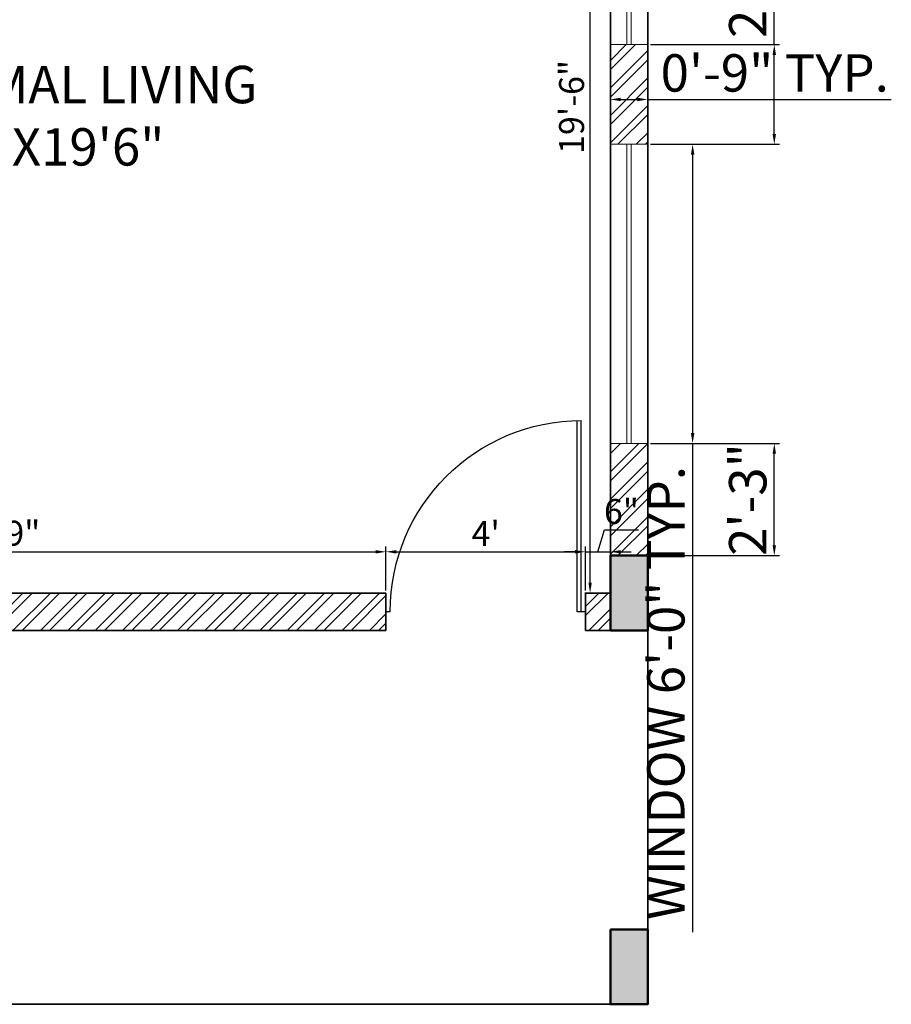
# Model space of a CAD drawing. Units: inches. Extents: x 4153 to 5577, y 785 to 1503.
# Tile 7 of 11: x 5367 to 5577, y 901 to 1138. Entities that reach past the tile are written whole.
import ezdxf

# ---------------------------------------------------------------- set-up
doc = ezdxf.new("R2010")
doc.units = ezdxf.units.IN
for name, color, linetype, lineweight in [('A-ANNO-DIMS', 2, 'Continuous', 18), ('A-AREA-IDEN', 7, 'Continuous', 25), ('A-COLS', 7, 'Continuous', 50), ('A-DOOR', 3, 'Continuous', 25), ('A-GLAZ', 4, 'Continuous', 18), ('A-WALL', 7, 'Continuous', 35)]:
    doc.layers.add(name, color=color, linetype=linetype, lineweight=lineweight)
doc.layers.add('A-WALL-PATT', color=251, linetype='Continuous', lineweight=13, true_color=0x636466)
doc.styles.get("Standard").update_dxf_attribs({"font": 'arial.ttf'})
doc.dimstyles.new('ISO-25', dxfattribs={"dimtxt": 9, "dimasz": 2.5, "dimexe": 1.25, "dimexo": 0.625, "dimtad": 1, "dimlunit": 3, "dimtxsty": 'Standard', "dimcen": 2.5, "dimadec": 0, "dimazin": 0, "dimtfac": 1, "dimtmove": 0, "dimatfit": 3, "dimfxl": 1, "dimarcsym": 0})

# ---------------------------------------------------------------- blocks, each defined once
blk = doc.blocks.new('D')
for p, q in [((1, 0), (1, 46)), ((2, 0), (2, 46)), ((0, 0), (2, 0)), ((47, 0), (48, 0))]:
    blk.add_line(p, q)
at = {"ltscale": 0.5}
blk.add_arc((1, 0), 46, 0, 90, dxfattribs=at)
blk = doc.blocks.new('*D55')
at = {"layer": 'A-ANNO-DIMS', "color": 0, "lineweight": -2, "transparency": 16777216}
for p, q in [((5266.25, 1001.11), (5266.25, 1011.66)), ((5268.75, 1010.41), (5452.75, 1010.41)), ((5455.25, 1001.11), (5455.25, 1011.66))]:
    blk.add_line(p, q, dxfattribs=at)
at = {"layer": 'A-ANNO-DIMS', "color": 0, "transparency": 16777216}
for points in [[(5268.75, 1010.82), (5268.75, 1009.99), (5266.25, 1010.41)], [(5452.75, 1010.82), (5452.75, 1009.99), (5455.25, 1010.41)]]:
    blk.add_solid(points, dxfattribs=at)
at = {"layer": 'Defpoints', "color": 0, "transparency": 16777216}
for p in [(5455.25, 1010.41), (5266.25, 1000.49), (5455.25, 1000.49)]:
    blk.add_point(p, dxfattribs=at)
at = {"layer": 'A-ANNO-DIMS', "color": 0, "transparency": 16777216, "insert": (5360.75, 1014.1), "char_height": 6, "attachment_point": 5}
blk.add_mtext('15\'-9"', dxfattribs=at)
blk = doc.blocks.new('*D56')
at = {"layer": 'A-ANNO-DIMS', "color": 0, "lineweight": -2, "transparency": 16777216}
for p, q in [((5455.25, 1001.11), (5455.25, 1011.66)), ((5457.75, 1010.41), (5500.75, 1010.41)), ((5503.25, 1001.11), (5503.25, 1011.66))]:
    blk.add_line(p, q, dxfattribs=at)
at = {"layer": 'A-ANNO-DIMS', "color": 0, "transparency": 16777216}
for points in [[(5457.75, 1010.82), (5457.75, 1009.99), (5455.25, 1010.41)], [(5500.75, 1010.82), (5500.75, 1009.99), (5503.25, 1010.41)]]:
    blk.add_solid(points, dxfattribs=at)
at = {"layer": 'Defpoints', "color": 0, "transparency": 16777216}
for p in [(5503.25, 1010.41), (5455.25, 1000.49), (5503.25, 1000.49)]:
    blk.add_point(p, dxfattribs=at)
at = {"layer": 'A-ANNO-DIMS', "color": 0, "transparency": 16777216, "insert": (5479.25, 1014.03), "char_height": 6, "attachment_point": 5}
blk.add_mtext("4'", dxfattribs=at)
blk = doc.blocks.new('*D57')
at = {"layer": 'A-ANNO-DIMS', "color": 0, "lineweight": -2, "transparency": 16777216}
for p, q in [((5506.25, 1010.41), (5507.83, 1015.66)), ((5507.83, 1015.66), (5516.01, 1015.66)), ((5500.75, 1010.41), (5498.25, 1010.41)), ((5503.25, 1001.11), (5503.25, 1011.66)), ((5503.25, 1010.41), (5509.25, 1010.41)), ((5503.25, 1010.41), (5509.25, 1010.41)), ((5509.25, 1001.11), (5509.25, 1011.66)), ((5511.75, 1010.41), (5514.25, 1010.41))]:
    blk.add_line(p, q, dxfattribs=at)
at = {"layer": 'A-ANNO-DIMS', "color": 0, "transparency": 16777216}
for points in [[(5500.75, 1010.82), (5500.75, 1009.99), (5503.25, 1010.41)], [(5511.75, 1010.82), (5511.75, 1009.99), (5509.25, 1010.41)]]:
    blk.add_solid(points, dxfattribs=at)
at = {"layer": 'Defpoints', "color": 0, "transparency": 16777216}
for p in [(5509.25, 1010.41), (5503.25, 1000.49), (5509.25, 1000.49)]:
    blk.add_point(p, dxfattribs=at)
at = {"layer": 'A-ANNO-DIMS', "color": 0, "transparency": 16777216, "insert": (5511.92, 1019.35), "char_height": 6, "attachment_point": 5}
blk.add_mtext('6"', dxfattribs=at)
blk = doc.blocks.new('*D58')
at = {"layer": 'A-ANNO-DIMS', "color": 0, "lineweight": -2, "transparency": 16777216}
for p, q in [((5508.63, 1234.49), (5503.13, 1234.49)), ((5504.38, 1002.99), (5504.38, 1231.99)), ((5508.63, 1000.49), (5503.13, 1000.49))]:
    blk.add_line(p, q, dxfattribs=at)
at = {"layer": 'A-ANNO-DIMS', "color": 0, "transparency": 16777216}
for points in [[(5503.97, 1231.99), (5504.8, 1231.99), (5504.38, 1234.49)], [(5503.97, 1002.99), (5504.8, 1002.99), (5504.38, 1000.49)]]:
    blk.add_solid(points, dxfattribs=at)
at = {"layer": 'Defpoints', "color": 0, "transparency": 16777216}
for p in [(5504.38, 1234.49), (5509.25, 1234.49), (5509.25, 1000.49)]:
    blk.add_point(p, dxfattribs=at)
at = {"layer": 'A-ANNO-DIMS', "color": 0, "transparency": 16777216, "insert": (5500.69, 1117.49), "char_height": 6, "attachment_point": 5, "rotation": 90}
blk.add_mtext('19\'-6"', dxfattribs=at)
blk = doc.blocks.new('WINDOW-72IN')
for p, q in [((0, 9), (0, 0)), ((72, 9), (72, 0)), ((0, 5), (72, 5)), ((0, 4), (72, 4))]:
    blk.add_line(p, q)
blk = doc.blocks.new('COL-9X18IN')
at = {"transparency": 33554687}
h = blk.add_hatch(color=256, dxfattribs=at)
h.dxf.hatch_style = 1
h.paths.add_polyline_path([(9, 18), (0, 18), (0, 0), (9, 0)])
blk.add_lwpolyline([(0, 18), (9, 18), (9, 0), (0, 0)], close=True)
blk = doc.blocks.new('*D104')
at = {"layer": 'A-ANNO-DIMS', "color": 0, "lineweight": -2, "transparency": 16777216}
for p, q in [((5518.88, 1108.49), (5530.3, 1108.49)), ((5529.05, 1105.99), (5529.05, 1038.99)), ((5518.88, 1036.49), (5530.3, 1036.49)), ((5529.05, 1036.49), (5529.05, 918.85))]:
    blk.add_line(p, q, dxfattribs=at)
at = {"layer": 'A-ANNO-DIMS', "color": 0, "transparency": 16777216}
for points in [[(5528.64, 1105.99), (5529.47, 1105.99), (5529.05, 1108.49)], [(5528.64, 1038.99), (5529.47, 1038.99), (5529.05, 1036.49)]]:
    blk.add_solid(points, dxfattribs=at)
at = {"layer": 'Defpoints', "color": 0, "transparency": 16777216}
for p in [(5518.25, 1108.49), (5518.25, 1036.49), (5529.05, 1036.49)]:
    blk.add_point(p, dxfattribs=at)
at = {"layer": 'A-ANNO-DIMS', "color": 0, "transparency": 16777216, "insert": (5523.77, 976.42), "char_height": 9, "attachment_point": 5, "rotation": 90}
blk.add_mtext('WINDOW 6\'-0" TYP.', dxfattribs=at)
blk = doc.blocks.new('*D105')
at = {"layer": 'A-ANNO-DIMS', "color": 0, "lineweight": -2, "transparency": 16777216}
for p, q in [((5509.25, 1109.11), (5509.25, 1120.54)), ((5511.75, 1119.29), (5515.75, 1119.29)), ((5518.25, 1109.11), (5518.25, 1120.54)), ((5518.25, 1119.29), (5576.86, 1119.29))]:
    blk.add_line(p, q, dxfattribs=at)
at = {"layer": 'A-ANNO-DIMS', "color": 0, "transparency": 16777216}
for points in [[(5511.75, 1119.71), (5511.75, 1118.87), (5509.25, 1119.29)], [(5515.75, 1119.71), (5515.75, 1118.87), (5518.25, 1119.29)]]:
    blk.add_solid(points, dxfattribs=at)
at = {"layer": 'Defpoints', "color": 0, "transparency": 16777216}
for p in [(5518.25, 1119.29), (5509.25, 1108.49), (5518.25, 1108.49)]:
    blk.add_point(p, dxfattribs=at)
at = {"layer": 'A-ANNO-DIMS', "color": 0, "transparency": 16777216, "insert": (5548.81, 1124.51), "char_height": 9, "attachment_point": 5}
blk.add_mtext('0\'-9" TYP.', dxfattribs=at)
blk = doc.blocks.new('*D153')
at = {"layer": 'A-ANNO-DIMS', "color": 0, "lineweight": -2, "transparency": 16777216}
for p, q in [((5518.88, 1036.49), (5549.95, 1036.49)), ((5548.7, 1011.99), (5548.7, 1033.99)), ((5518.88, 1009.49), (5549.95, 1009.49))]:
    blk.add_line(p, q, dxfattribs=at)
at = {"layer": 'A-ANNO-DIMS', "color": 0, "transparency": 16777216}
for points in [[(5548.29, 1033.99), (5549.12, 1033.99), (5548.7, 1036.49)], [(5548.29, 1011.99), (5549.12, 1011.99), (5548.7, 1009.49)]]:
    blk.add_solid(points, dxfattribs=at)
at = {"layer": 'Defpoints', "color": 0, "transparency": 16777216}
for p in [(5518.25, 1036.49), (5548.7, 1036.49), (5518.25, 1009.49)]:
    blk.add_point(p, dxfattribs=at)
at = {"layer": 'A-ANNO-DIMS', "color": 0, "transparency": 16777216, "insert": (5543.48, 1022.99), "char_height": 9, "attachment_point": 5, "rotation": 90}
blk.add_mtext('2\'-3"', dxfattribs=at)
blk = doc.blocks.new('*D154')
at = {"layer": 'A-ANNO-DIMS', "color": 0, "lineweight": -2, "transparency": 16777216}
for p, q in [((5548.7, 1132.49), (5548.7, 1160.32)), ((5518.88, 1132.49), (5549.95, 1132.49)), ((5548.7, 1110.99), (5548.7, 1129.99)), ((5518.88, 1108.49), (5549.95, 1108.49))]:
    blk.add_line(p, q, dxfattribs=at)
at = {"layer": 'A-ANNO-DIMS', "color": 0, "transparency": 16777216}
for points in [[(5548.29, 1129.99), (5549.12, 1129.99), (5548.7, 1132.49)], [(5548.29, 1110.99), (5549.12, 1110.99), (5548.7, 1108.49)]]:
    blk.add_solid(points, dxfattribs=at)
at = {"layer": 'Defpoints', "color": 0, "transparency": 16777216}
for p in [(5518.25, 1132.49), (5548.7, 1132.49), (5518.25, 1108.49)]:
    blk.add_point(p, dxfattribs=at)
at = {"layer": 'A-ANNO-DIMS', "color": 0, "transparency": 16777216, "insert": (5543.48, 1147.65), "char_height": 9, "attachment_point": 5, "rotation": 90}
blk.add_mtext('2\'-0"', dxfattribs=at)

msp = doc.modelspace()

# ---------------------------------------------------------------- hatches: boundary and pattern name
at = {"layer": 'A-WALL-PATT', "transparency": 33554687}
h = msp.add_hatch(dxfattribs=at)
h.set_pattern_fill('ANSI32', color=256, scale=0.49)
h.set_pattern_definition([(45, (816.3263, 0), (-3.300244, 3.300244), []), (45, (818.5265, 0), (-3.300244, 3.300244), [])])
h.paths.add_polyline_path([(5011.254, 1088.988), (5020.254, 1088.988), (5020.254, 1129.488), (5155.254, 1129.488), (5155.254, 1105.488), (5161.254, 1105.488), (5161.254, 1138.488), (5098.254, 1138.488), (5098.254, 1234.488), (5113.254, 1234.488), (5113.254, 1243.488), (5086.254, 1243.488), (5086.254, 1234.488), (5092.254, 1234.488), (5092.254, 1138.488), (5020.254, 1138.488), (5020.254, 1168.488), (5011.254, 1168.488)])
h.paths.add_polyline_path([(5011.254, 1009.488), (5020.254, 1009.488), (5020.254, 1040.988), (5011.254, 1040.988)])
h.paths.add_polyline_path([(5095.254, 991.488), (5095.254, 1000.488), (5020.254, 1000.488), (5020.254, 991.488)])
h.paths.add_polyline_path([(5011.254, 910.488), (5020.254, 910.488), (5020.254, 991.488), (5011.254, 991.488)])
h.paths.add_polyline_path([(5152.254, 901.488), (5152.254, 907.488), (5020.254, 907.488), (5020.254, 901.488)])
h.paths.add_polyline_path([(5161.254, 1057.488), (5155.254, 1057.488), (5155.254, 1000.488), (5161.254, 1000.488)])
h.paths.add_polyline_path([(5143.254, 991.488), (5152.254, 991.488), (5152.254, 1000.488), (5143.254, 1000.488)])
h.paths.add_polyline_path([(5161.254, 1000.488), (5161.254, 991.488), (5185.254, 991.488), (5185.254, 1000.488)])
h.paths.add_polyline_path([(5257.254, 991.488), (5257.254, 1000.488), (5233.254, 1000.488), (5233.254, 991.488)])
h.paths.add_polyline_path([(5266.254, 1120.488), (5257.254, 1120.488), (5257.254, 1000.488), (5266.254, 1000.488)])
h.paths.add_polyline_path([(5290.254, 991.488), (5290.254, 1000.488), (5275.254, 1000.488), (5275.254, 991.488)])
h.paths.add_polyline_path([(5362.254, 1000.488), (5362.254, 991.488), (5455.254, 991.488), (5455.254, 1000.488)])
h.paths.add_polyline_path([(5509.254, 1009.488), (5518.254, 1009.488), (5518.254, 1036.488), (5509.254, 1036.488)])
h.paths.add_polyline_path([(5503.254, 1000.488), (5503.254, 991.488), (5509.254, 991.488), (5509.254, 1000.488)])
h.paths.add_polyline_path([(5518.254, 1132.488), (5509.254, 1132.488), (5509.254, 1108.488), (5518.254, 1108.488)])
h.paths.add_polyline_path([(5509.254, 1204.488), (5518.254, 1204.488), (5518.254, 1225.488), (5509.254, 1225.488)])
h.paths.add_polyline_path([(5467.254, 1234.488), (5467.254, 1243.488), (5377.254, 1243.488), (5377.254, 1265.228), (5377.254, 1381.488), (5467.254, 1381.488), (5467.254, 1393.488), (5461.254, 1393.488), (5461.254, 1387.488), (5377.254, 1387.488), (5377.254, 1435.488), (5368.254, 1435.488), (5368.254, 1354.488), (5347.254, 1354.488), (5347.254, 1348.488), (5368.254, 1348.488), (5368.254, 1309.488), (5302.254, 1309.488), (5302.254, 1234.488), (5321.754, 1234.488), (5321.754, 1243.488), (5311.254, 1243.488), (5311.254, 1303.488), (5368.254, 1303.488), (5368.254, 1243.488), (5357.754, 1243.488), (5357.754, 1234.488)])
h.paths.add_polyline_path([(5509.254, 1357.488), (5518.254, 1357.488), (5518.254, 1426.488), (5509.254, 1426.488)])
h.paths.add_polyline_path([(5509.254, 1243.488), (5518.254, 1243.488), (5518.254, 1309.488), (5509.254, 1309.488)])
h.paths.add_polyline_path([(5509.254, 1435.488), (5509.254, 1444.488), (5425.254, 1444.488), (5425.254, 1435.488), (5461.254, 1435.488), (5461.254, 1423.488), (5467.254, 1423.488), (5467.254, 1435.488)])
h.paths.add_polyline_path([(5302.254, 1435.488), (5302.254, 1348.488), (5317.254, 1348.488), (5317.254, 1354.488), (5311.254, 1354.488), (5311.254, 1435.488), (5314.254, 1435.488), (5314.254, 1444.488), (5296.254, 1444.488), (5296.254, 1435.488)])
h.paths.add_polyline_path([(5368.254, 1444.488), (5362.254, 1444.488), (5362.254, 1435.488), (5368.254, 1435.488)])
h.paths.add_polyline_path([(5389.254, 1444.488), (5386.254, 1444.488), (5386.254, 1435.488), (5389.254, 1435.488)])
h.paths.add_polyline_path([(5248.254, 1435.488), (5248.254, 1444.488), (5173.254, 1444.488), (5173.254, 1435.488)])
h.paths.add_polyline_path([(5101.254, 1435.488), (5101.254, 1444.488), (5020.254, 1444.488), (5020.254, 1435.488)])
h.paths.add_polyline_path([(5011.254, 1293.488), (5020.254, 1293.488), (5020.254, 1295.242), (5020.254, 1426.488), (5011.254, 1426.488)])
h.paths.add_polyline_path([(5155.254, 1243.488), (5149.254, 1243.488), (5149.254, 1234.488), (5248.254, 1234.488), (5248.254, 1243.488), (5164.254, 1243.488), (5164.254, 1435.488), (5155.254, 1435.488)])
h.paths.add_polyline_path([(5020.254, 1243.488), (5020.254, 1234.488), (5056.254, 1234.488), (5056.254, 1243.488)], flags=17)
h.paths.add_polyline_path([(5020.254, 1225.488), (5011.254, 1225.488), (5011.254, 1198.488), (5020.254, 1198.488)], flags=17)

# ---------------------------------------------------------------- linework, layer by layer
at = {"layer": 'A-WALL'}
for p, q in [((5518.254, 1444.488), (5518.254, 901.488)), ((5509.254, 1234.488), (5509.254, 1000.488)), ((5266.254, 1000.488), (5455.254, 1000.488)), ((5455.254, 1000.488), (5455.254, 991.488)), ((5503.254, 1000.488), (5509.254, 1000.488)), ((5503.254, 1000.488), (5503.254, 991.488)), ((5020.254, 991.488), (5455.254, 991.488)), ((5503.254, 991.488), (5518.254, 991.488)), ((5518.254, 901.488), (5011.254, 901.488))]:
    msp.add_line(p, q, dxfattribs=at)

# ---------------------------------------------------------------- block references
at = {"layer": 'A-COLS'}
for p in [(5509.254, 991.488), (5509.254, 901.488)]:
    msp.add_blockref('COL-9X18IN', p, dxfattribs=at)
at = {"layer": 'A-DOOR', "xscale": -1}
msp.add_blockref('D', (5503.254, 995.988), dxfattribs=at)
at = {"layer": 'A-GLAZ'}
for p, rotation in [((5509.254, 1204.488), 269.9999999999994), ((5509.254, 1108.488), 270.0000000000009)]:
    msp.add_blockref('WINDOW-72IN', p, dxfattribs=dict(at, rotation=rotation))

# ---------------------------------------------------------------- texts
at = {"layer": 'A-AREA-IDEN', "insert": (5335.538, 1127.378), "char_height": 9, "attachment_point": 1}
msp.add_mtext_dynamic_manual_height_columns('{\\fTimes New Roman|b0|i0|c0|p18;FORMAL LIVING\\P20\'3"X19\'6"}', width=119.83324, gutter_width=12.5, heights=[0], dxfattribs=at)

# ---------------------------------------------------------------- dimensions: what is measured, and where the dimension line sits
at = {"layer": 'A-ANNO-DIMS'}
for base, p1, p2, override, picture, middle in [((5504.382, 1234.488), (5509.254, 1000.488), (5509.254, 1234.488), {"dimtxt": 6, "dimclrd": 0, "dimclre": 0, "dimclrt": 0}, '*D58', (5500.693, 1117.488)), ((5548.704, 1132.488), (5518.254, 1108.488), (5518.254, 1132.488), {"dimdec": 1, "dimlfac": 1, "dimrnd": 0, "dimzin": 1, "dimdsep": 46, "dimlunit": 4, "dimfrac": 2}, '*D154', (5543.484, 1147.652)), ((5548.704, 1036.488), (5518.254, 1009.488), (5518.254, 1036.488), {"dimdec": 1, "dimlfac": 1, "dimrnd": 0, "dimzin": 1, "dimdsep": 46, "dimlunit": 4, "dimfrac": 2}, '*D153', (5543.481, 1022.988))]:
    dim = msp.add_linear_dim(base=base, p1=p1, p2=p2, angle=90, dimstyle='ISO-25', override=override, dxfattribs=at)
    dim.commit()
    dim.dimension.update_dxf_attribs({"geometry": picture, "text_midpoint": middle})
for base, p1, p2, angle, text, picture, middle in [((5518.254, 1119.288), (5509.254, 1108.488), (5518.254, 1108.488), 0, '<> TYP.', '*D105', (5548.809, 1124.509)), ((5529.054, 1036.488), (5518.254, 1108.488), (5518.254, 1036.488), 270, 'WINDOW <> TYP.', '*D104', (5523.772, 976.42))]:
    dim = msp.add_linear_dim(base=base, p1=p1, p2=p2, angle=angle, text=text, dimstyle='ISO-25', override={"dimdec": 1, "dimlfac": 1, "dimrnd": 0, "dimzin": 1, "dimdsep": 46, "dimlunit": 4, "dimfrac": 2}, dxfattribs=at)
    dim.commit()
    dim.dimension.update_dxf_attribs({"geometry": picture, "text_midpoint": middle})
for base, p1, p2, override, picture, middle in [((5509.254, 1010.407), (5503.254, 1000.488), (5509.254, 1000.488), {"dimtxt": 6, "dimclrd": 0, "dimclre": 0, "dimclrt": 0, "dimtmove": 1}, '*D57', (5508.454, 1019.346)), ((5455.254, 1010.407), (5266.254, 1000.488), (5455.254, 1000.488), {"dimtxt": 6, "dimclrd": 0, "dimclre": 0, "dimclrt": 0}, '*D55', (5360.754, 1014.095)), ((5503.254, 1010.407), (5455.254, 1000.488), (5503.254, 1000.488), {"dimtxt": 6, "dimclrd": 0, "dimclre": 0, "dimclrt": 0, "dimtmove": 1}, '*D56', (5479.254, 1014.032))]:
    dim = msp.add_linear_dim(base=base, p1=p1, p2=p2, dimstyle='ISO-25', override=override, dxfattribs=at)
    dim.commit()
    dim.dimension.update_dxf_attribs({"geometry": picture, "text_midpoint": middle})

doc.saveas('drawing.dxf')
